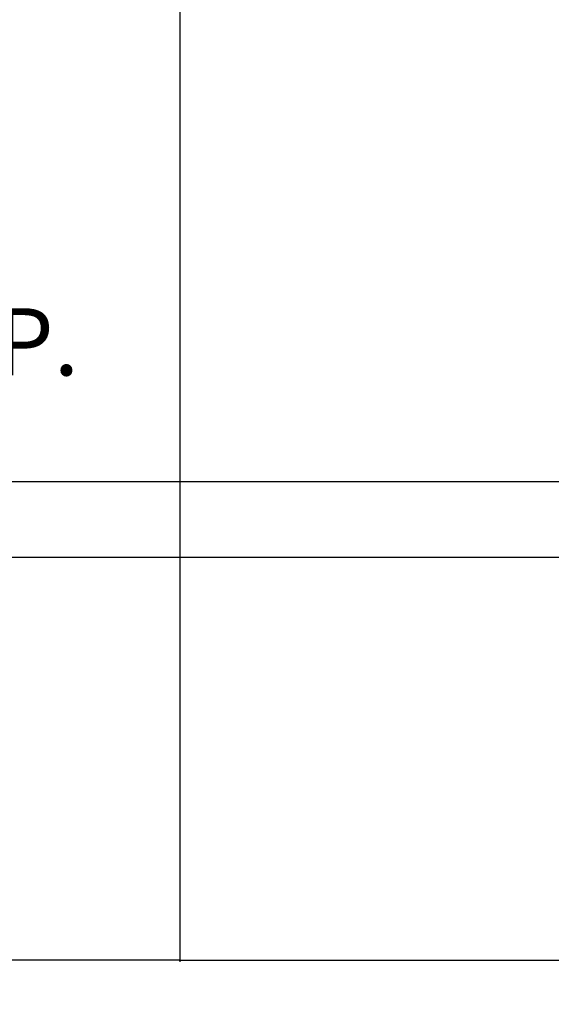
# Model space of a CAD drawing. Units: inches. Extents: x -48 to 50072, y 0 to 21068.
# Tile 9 of 75: x 278 to 341, y 161 to 278. Entities that reach past the tile are written whole.
import ezdxf

# ---------------------------------------------------------------- set-up
doc = ezdxf.new("R2010")
doc.units = ezdxf.units.IN
doc.header["$MEASUREMENT"] = 0
doc.layers.add('A-ANNO-DIMS', color=2, linetype='Continuous', lineweight=18)
doc.layers.add('C-PROP', color=7, linetype='Continuous', lineweight=25)
doc.styles.get("Standard").update_dxf_attribs({"font": 'arial.ttf'})
doc.dimstyles.get("Standard").update_dxf_attribs({"dimtxt": 8, "dimasz": 0.18, "dimexe": 0.18, "dimexo": 0.0625, "dimgap": 0.09, "dimtad": 0, "dimtih": 1, "dimtoh": 1, "dimdec": 1, "dimzin": 0, "dimdsep": 46, "dimlunit": 4, "dimtxsty": 'Standard', "dimblk": 'ARCHTICK', "dimcen": 0.09, "dimadec": 0, "dimazin": 0, "dimtfac": 1, "dimtdec": 1, "dimtofl": 0, "dimtmove": 0, "dimatfit": 3, "dimldrblk": 'ARCHTICK', "dimfxl": 1, "dimtolj": 1, "dimtzin": 0, "dimarcsym": 0})

# ---------------------------------------------------------------- blocks, each defined once
blk = doc.blocks.new('_ArchTick')
at = {"color": 0, "linetype": 'ByBlock', "const_width": 0.15}
blk.add_lwpolyline([(-0.5, -0.5), (0.5, 0.5)], dxfattribs=at)
blk = doc.blocks.new('*D52')
at = {"layer": 'A-ANNO-DIMS', "color": 0, "lineweight": -2, "transparency": 16777216}
for p, q in [((238.85, 252.65), (242.86, 252.65)), ((242.68, 252.65), (242.68, 243.9)), ((242.68, 226.69), (242.68, 235.44)), ((238.85, 226.69), (242.86, 226.69))]:
    blk.add_line(p, q, dxfattribs=at)
at = {"layer": 'Defpoints', "color": 0, "transparency": 16777216}
for p in [(238.78, 252.65), (242.68, 252.65), (238.78, 226.69)]:
    blk.add_point(p, dxfattribs=at)
at = {"layer": 'A-ANNO-DIMS', "color": 0, "lineweight": -2, "transparency": 16777216, "xscale": 0.18, "yscale": 0.18, "zscale": 0.18}
for p, rotation in [((242.68, 252.65), 90), ((242.68, 226.69), 270)]:
    blk.add_blockref('_ArchTick', p, dxfattribs=dict(at, rotation=rotation))
at = {"layer": 'A-ANNO-DIMS', "color": 0, "transparency": 16777216, "insert": (242.68, 239.67), "char_height": 8, "attachment_point": 5}
blk.add_mtext('\\A1;SHRUB A 26 TYP.', dxfattribs=at)
blk = doc.blocks.new('*D117')
at = {"layer": 'A-ANNO-DIMS', "color": 0, "lineweight": -2, "transparency": 16777216}
for p, q in [((216.02, 488.71), (216.02, 165.94)), ((297.02, 488.71), (297.02, 165.94)), ((216.02, 166.12), (251.46, 166.12)), ((297.02, 166.12), (261.57, 166.12))]:
    blk.add_line(p, q, dxfattribs=at)
at = {"layer": 'Defpoints', "color": 0, "transparency": 16777216}
for p in [(216.02, 488.77), (297.02, 488.77), (297.02, 166.12)]:
    blk.add_point(p, dxfattribs=at)
at = {"layer": 'A-ANNO-DIMS', "color": 0, "lineweight": -2, "transparency": 16777216, "xscale": 0.18, "yscale": 0.18, "zscale": 0.18, "rotation": 180}
blk.add_blockref('_ArchTick', (216.02, 166.12), dxfattribs=at)
at = {"layer": 'A-ANNO-DIMS', "color": 0, "lineweight": -2, "transparency": 16777216, "xscale": 0.18, "yscale": 0.18, "zscale": 0.18}
blk.add_blockref('_ArchTick', (297.02, 166.12), dxfattribs=at)
at = {"layer": 'A-ANNO-DIMS', "color": 0, "transparency": 16777216, "insert": (256.52, 166.12), "char_height": 8, "attachment_point": 5}
blk.add_mtext('\\A1;81', dxfattribs=at)
blk = doc.blocks.new('*D118')
at = {"layer": 'A-ANNO-DIMS', "color": 0, "lineweight": -2, "transparency": 16777216}
for p, q in [((297.02, 488.71), (297.02, 165.94)), ((463.52, 488.71), (463.52, 165.94)), ((297.02, 166.12), (367.03, 166.12)), ((463.52, 166.12), (393.51, 166.12))]:
    blk.add_line(p, q, dxfattribs=at)
at = {"layer": 'Defpoints', "color": 0, "transparency": 16777216}
for p in [(297.02, 488.77), (463.52, 488.77), (463.52, 166.12)]:
    blk.add_point(p, dxfattribs=at)
at = {"layer": 'A-ANNO-DIMS', "color": 0, "lineweight": -2, "transparency": 16777216, "xscale": 0.18, "yscale": 0.18, "zscale": 0.18, "rotation": 180}
blk.add_blockref('_ArchTick', (297.02, 166.12), dxfattribs=at)
at = {"layer": 'A-ANNO-DIMS', "color": 0, "lineweight": -2, "transparency": 16777216, "xscale": 0.18, "yscale": 0.18, "zscale": 0.18}
blk.add_blockref('_ArchTick', (463.52, 166.12), dxfattribs=at)
at = {"layer": 'A-ANNO-DIMS', "color": 0, "transparency": 16777216, "insert": (380.27, 166.12), "char_height": 8, "attachment_point": 5}
blk.add_mtext('\\A1;166.5', dxfattribs=at)

msp = doc.modelspace()

# ---------------------------------------------------------------- linework, layer by layer
at = {"layer": 'C-PROP'}
for p, q in [((210.389, 223.075), (544.517, 223.075)), ((210.389, 214.075), (553.517, 214.075))]:
    msp.add_line(p, q, dxfattribs=at)

# ---------------------------------------------------------------- dimensions: what is measured, and where the dimension line sits
at = {"layer": 'A-ANNO-DIMS'}
for base, p1, p2, override, picture, middle in [((297.017, 166.125), (216.017, 488.775), (297.017, 488.775), {"dimdec": 0, "dimlfac": 1, "dimrnd": 0, "dimzin": 0, "dimdsep": 46, "dimlunit": 2}, '*D117', (256.517, 166.125)), ((463.517, 166.125), (297.017, 488.775), (463.517, 488.775), {"dimdec": 1, "dimlfac": 1, "dimrnd": 0, "dimzin": 0, "dimdsep": 46, "dimlunit": 2}, '*D118', (380.267, 166.125))]:
    dim = msp.add_linear_dim(base=base, p1=p1, p2=p2, dimstyle='Standard', override=override, dxfattribs=at)
    dim.commit()
    dim.dimension.update_dxf_attribs({"geometry": picture, "text_midpoint": middle})
dim = msp.add_linear_dim(base=(242.679, 252.654), p1=(238.784, 226.686), p2=(238.784, 252.654), angle=90, text='SHRUB A <> TYP.', dimstyle='Standard', override={"dimdec": 0, "dimlfac": 1, "dimrnd": 0, "dimzin": 0, "dimdsep": 46, "dimlunit": 2}, dxfattribs=at)
dim.commit()
dim.dimension.update_dxf_attribs({"geometry": '*D52', "text_midpoint": (242.679, 239.67)})

doc.saveas('drawing.dxf')
